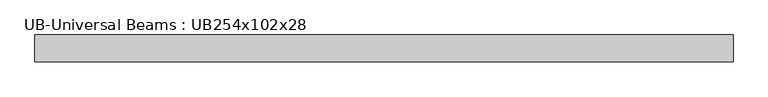
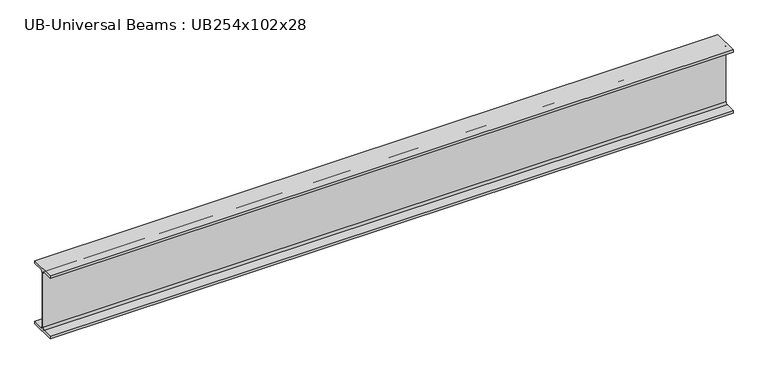
"""IFC4 building model written with IfcOpenShell, lengths in millimetres: beam geometry, UB-Universal Beams : UB254x102x28."""

from ifc_helpers import new_model, si_unit, point, frame, frame_2d, origin, place, context, project, spatial, polyline, circle_curve, trimmed, segment, composite_curve, outline, extrude, source, transform, mapped, element, save


def ub_universal_beams_ub254x102x28_1dca85a9(model_context):
    return source(origin(), model_context, "Body", "SweptSolid", [
        extrude(outline(composite_curve([segment(polyline([(51.1, -120.2), (51.1, -130.2), (-51.1, -130.2), (-51.1, -120.2), (-10.75, -120.2)]), True, "CONTINUOUS"), segment(trimmed(circle_curve(frame_2d((-10.75, -112.6)), 7.6), [point((-10.75, -120.2))], [point((-3.15, -112.6))], True, "CARTESIAN"), True, "CONTINUOUS"), segment(polyline([(-3.15, -112.6), (-3.15, 112.6)]), True, "CONTINUOUS"), segment(trimmed(circle_curve(frame_2d((-10.75, 112.6)), 7.6), [point((-3.15, 112.6))], [point((-10.75, 120.2))], True, "CARTESIAN"), True, "CONTINUOUS"), segment(polyline([(-10.75, 120.2), (-51.1, 120.2), (-51.1, 130.2), (51.1, 130.2), (51.1, 120.2), (10.75, 120.2)]), True, "CONTINUOUS"), segment(trimmed(circle_curve(frame_2d((10.75, 112.6)), 7.6), [point((10.75, 120.2))], [point((3.15, 112.6))], True, "CARTESIAN"), True, "CONTINUOUS"), segment(polyline([(3.15, 112.6), (3.15, -112.6)]), True, "CONTINUOUS"), segment(trimmed(circle_curve(frame_2d((10.75, -112.6)), 7.6), [point((3.15, -112.6))], [point((10.75, -120.2))], True, "CARTESIAN"), True, "CONTINUOUS"), segment(polyline([(10.75, -120.2), (51.1, -120.2)]), True, "CONTINUOUS")], self_intersect=False)), frame((-1381.1, 0.0, 0.0), z_axis=(1.0, 0.0, 0.0), x_axis=(0.0, 1.0, 0.0)), (0.0, 0.0, 1.0), 2666.2),
    ])


if __name__ == "__main__":
    model = new_model("IFC4")
    model_context = context("Model", 3, world=origin())
    ifc_project = project(units=[si_unit("LENGTHUNIT", "METRE", prefix="MILLI")], contexts=[model_context])
    site = spatial("IfcSite", under=ifc_project)
    building = spatial("IfcBuilding", under=site)
    placement = place(None, origin())
    ub_universal_beams_ub254x102x28_shape = ub_universal_beams_ub254x102x28_1dca85a9(model_context)
    element("IfcBeam", 1, ObjectType="UB-Universal Beams : UB254x102x28", at=placement, inside=building, context=model_context, shape_type="MappedRepresentation", body=[
        mapped(ub_universal_beams_ub254x102x28_shape, transform((0.0, 0.0, 0.0), x_axis=(1.0, 0.0, 0.0), y_axis=(0.0, 1.0, 0.0), z_axis=(0.0, 0.0, 1.0))),
    ])
    save(model, "model.ifc")

# Revit data of these elements
# Type "UB-Universal Beams : UB254x102x28"
#   Section Name Key = "UB254X102X28"
#   Width = 10.22 cm
#   Web Thickness = 0.63 cm
#   Web Fillet = 0.76 cm
#   Warping Constant = 28000.0 cm⁶
#   Torsional Moment of Inertia = 9.57 cm⁴
#   Section Area = 36.1 cm²
#   Plastic Modulus weak axis = 54.8 cm³
#   Plastic Modulus strong axis = 353.0 cm³
#   Nominal Weight = 28.2999 kgf/m
#   Moment of Inertia weak axis = 179.00 cm⁴
#   Moment of Inertia strong axis = 4005.00 cm⁴
#   Height = 26.04 cm
#   Flange Thickness = 1.0 cm
#   Elastic Modulus weak axis = 34.9 cm³
#   Elastic Modulus strong axis = 308.0 cm³
#   Centroid Vertical = 13.02 cm
#   Centroid Horizontal = 5.11 cm
#   Bolt Spacing = 5.4 cm
#   Length [instance default] = 4' - 11.05512"
#   Structural Material [instance default] = Metal - Steel 43-275
#   Type Comments = ""
#   Assembly Code = ""
# Element 1 (IfcBeam, "UB-Universal Beams : UB254x102x28")
#   Materials on its faces: "Metal - Steel 43-275"
# Materials
#   "Metal - Steel 43-275": class "Metal", colour RGB 247 247 247, transparency 0, Cost = 0
